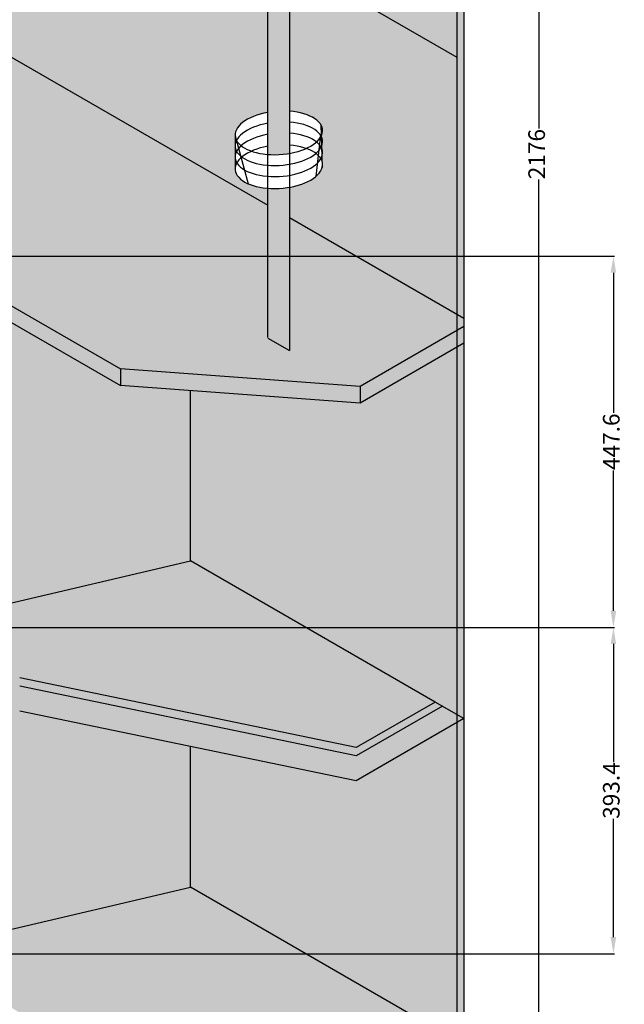
# Model space of a CAD drawing. Units: millimetres. Extents: x 78378 to 86415, y 148682 to 152721.
# Tile 11 of 18: x 81240 to 81968, y 149308 to 150495. Entities that reach past the tile are written whole.
import ezdxf

# ---------------------------------------------------------------- set-up
doc = ezdxf.new("R2010")
doc.units = ezdxf.units.MM
for name, color, linetype, lineweight in [('A-ANNO-DIMS', 2, 'Continuous', 18), ('A-FURN', 4, 'Continuous', 25), ('A-FURN-PATT', 32, 'Continuous', 13)]:
    doc.layers.add(name, color=color, linetype=linetype, lineweight=lineweight)
doc.styles.get("Standard").update_dxf_attribs({"font": 'arial.ttf'})
doc.dimstyles.new('ISO-25', dxfattribs={"dimtxt": 20, "dimasz": 20, "dimexe": 1.25, "dimexo": 0.625, "dimtad": 0, "dimdec": 1, "dimtxsty": 'Standard', "dimcen": 2.5, "dimadec": 0, "dimazin": 0, "dimtfac": 1, "dimtdec": 1, "dimtmove": 0, "dimatfit": 3, "dimfxl": 1, "dimarcsym": 0})

# ---------------------------------------------------------------- blocks, each defined once
blk = doc.blocks.new('*D1')
at = {"layer": 'A-ANNO-DIMS', "color": 0, "lineweight": -2, "transparency": 16777216}
for p, q in [((81775.8, 151435), (81866.6, 151435)), ((81865.3, 151415), (81865.3, 150363.7)), ((81865.3, 149279), (81865.3, 150302.4)), ((81775.8, 149259), (81866.6, 149259))]:
    blk.add_line(p, q, dxfattribs=at)
at = {"layer": 'A-ANNO-DIMS', "color": 0, "transparency": 16777216}
for points in [[(81862, 151415), (81868.6, 151415), (81865.3, 151435)], [(81862, 149279), (81868.6, 149279), (81865.3, 149259)]]:
    blk.add_solid(points, dxfattribs=at)
at = {"layer": 'Defpoints', "color": 0, "transparency": 16777216}
for p in [(81775.2, 151435), (81775.2, 149259), (81865.3, 149259)]:
    blk.add_point(p, dxfattribs=at)
at = {"layer": 'A-ANNO-DIMS', "color": 0, "transparency": 16777216, "insert": (81865.3, 150333), "char_height": 20, "attachment_point": 5, "rotation": 90}
blk.add_mtext('2176', dxfattribs=at)
blk = doc.blocks.new('*D28')
at = {"layer": 'A-ANNO-DIMS', "color": 0, "lineweight": -2, "transparency": 16777216}
for p, q in [((81117.6, 149762.4), (81956.4, 149762.4)), ((81955.2, 149742.4), (81955.2, 149600)), ((81955.2, 149389), (81955.2, 149531.4)), ((81117.6, 149369), (81956.4, 149369))]:
    blk.add_line(p, q, dxfattribs=at)
at = {"layer": 'A-ANNO-DIMS', "color": 0, "transparency": 16777216}
for points in [[(81951.8, 149742.4), (81958.5, 149742.4), (81955.2, 149762.4)], [(81951.8, 149389), (81958.5, 149389), (81955.2, 149369)]]:
    blk.add_solid(points, dxfattribs=at)
at = {"layer": 'Defpoints', "color": 0, "transparency": 16777216}
for p in [(81117, 149762.4), (81955.2, 149762.4), (81117, 149369)]:
    blk.add_point(p, dxfattribs=at)
at = {"layer": 'A-ANNO-DIMS', "color": 0, "transparency": 16777216, "insert": (81955.2, 149565.7), "char_height": 20, "attachment_point": 5, "rotation": 90}
blk.add_mtext('393.4', dxfattribs=at)
blk = doc.blocks.new('*D29')
at = {"layer": 'A-ANNO-DIMS', "color": 0, "lineweight": -2, "transparency": 16777216}
for p, q in [((81126.3, 150210), (81956.4, 150210)), ((81955.2, 150190), (81955.2, 150021)), ((81955.2, 149782.4), (81955.2, 149951.4)), ((81117.6, 149762.4), (81956.4, 149762.4))]:
    blk.add_line(p, q, dxfattribs=at)
at = {"layer": 'A-ANNO-DIMS', "color": 0, "transparency": 16777216}
for points in [[(81951.8, 150190), (81958.5, 150190), (81955.2, 150210)], [(81951.8, 149782.4), (81958.5, 149782.4), (81955.2, 149762.4)]]:
    blk.add_solid(points, dxfattribs=at)
at = {"layer": 'Defpoints', "color": 0, "transparency": 16777216}
for p in [(81125.6, 150210), (81955.2, 150210), (81117, 149762.4)]:
    blk.add_point(p, dxfattribs=at)
at = {"layer": 'A-ANNO-DIMS', "color": 0, "transparency": 16777216, "insert": (81955.2, 149986.2), "char_height": 20, "attachment_point": 5, "rotation": 90}
blk.add_mtext('447.6', dxfattribs=at)

msp = doc.modelspace()

# ---------------------------------------------------------------- hatches: boundary and pattern name
at = {"layer": 'A-FURN-PATT'}
h = msp.add_hatch(color=256, dxfattribs=at)
h.dxf.hatch_style = 1
h.paths.add_polyline_path([(78839.3276, 151040.0076), (78579.52, 151190.0076), (78579.52, 150470.0076), (78839.3276, 150320.0076)])
h.paths.add_polyline_path([(79073.1545, 150899.6469, 0.277779695), (79002.2645, 150996.3205, 0.791083931), (78917.9567, 150978.8719, 0.180448316), (78856.6481, 150853.0138), (78856.6481, 150350.6973), (79073.1545, 150484.318)])
h.paths.add_polyline_path([(79073.1545, 151175.0076), (78856.6481, 151050.0076), (78856.6481, 150853.0138, -0.180448316), (78917.9567, 150978.8719, -0.791083931), (79002.2645, 150996.3205, -0.277779695), (79073.1545, 150899.6469)])
h.paths.add_polyline_path([(79341.6224, 151350.0076), (79099.1352, 151490.0076), (78596.8405, 151200.0076), (78839.3276, 151060.0076)])
h.paths.add_polyline_path([(79904.5389, 151675.0076), (79662.0518, 151815.0076), (79099.1352, 151490.0076), (79341.6224, 151350.0076)])
h.paths.add_polyline_path([(80389.5131, 151955.0076), (80389.5131, 152235.0076), (79662.0518, 151815.0076), (79904.5389, 151675.0076)])
h.paths.add_polyline_path([(80389.5131, 151955.0076), (80164.3465, 151825.0076), (80164.3465, 151105.0076), (80614.6797, 151105.0076), (80614.6797, 151825.0076)])
edge = h.paths.add_edge_path(flags=16)
edge.add_spline(control_points=[(80216.308, 151728.251), (80227.1854, 151732.981), (80256.3301, 151745.6544), (80298.41, 151761.9595), (80340.2597, 151805.855), (80391.0771, 151782.0404), (80454.0396, 151805.7581), (80496.5007, 151742.4095), (80543.8218, 151733.4043), (80562.7182, 151729.8083)], knot_values=[0, 0, 0, 0, 35.543746761, 95.235753469, 136.367675126, 200.932981967, 236.726410811, 322.889934976, 380.170273667, 380.170273667, 380.170273667, 380.170273667], degree=3, periodic=0)
edge.add_line((80562.7182, 151729.8083), (80562.7182, 151165.0076))
edge.add_line((80562.7182, 151165.0076), (80216.308, 151165.0076))
edge.add_line((80216.308, 151165.0076), (80216.308, 151728.251))
h.paths.add_polyline_path([(80632.0002, 152095.0076), (80389.5131, 152235.0076), (80389.5131, 151955.0076), (80614.6797, 151825.0076), (80632.0002, 151815.0076)])
h.paths.add_polyline_path([(80867.7794, 151958.8805), (80632.0002, 152095.0076), (80632.0002, 151815.0076), (80632.0002, 151510.0076), (80867.7794, 151373.8805)])
h.paths.add_polyline_path([(80147.026, 151495.8203, 0.18918979), (80063.5671, 151597.7244, 0.788261355), (79979.2691, 151580.5832, 0.160726132), (79904.5389, 151413.5769), (79904.5389, 150955.0076), (80147.026, 151095.0076)])
h.paths.add_polyline_path([(80147.026, 151815.0076), (79904.5389, 151675.0076), (79904.5389, 151413.5769, -0.160726132), (79979.2691, 151580.5832, -0.788261355), (80063.5671, 151597.7244, -0.18918979), (80147.026, 151495.8203)])
h.paths.add_polyline_path([(79887.2184, 151645.0076), (79640.4011, 151502.5076), (79640.4011, 151262.3325, -0.160726132), (79715.1313, 151429.3387, -0.788261355), (79799.4294, 151446.48, -0.21290578), (79887.2184, 151328.7247)])
h.paths.add_polyline_path([(79799.4294, 151446.48, 0.788261355), (79715.1313, 151429.3387, 0.160726132), (79640.4011, 151262.3325), (79640.4011, 150822.5076), (79887.2184, 150965.0076), (79887.2184, 151328.7247, 0.21290578)])
h.paths.add_polyline_path([(79605.7601, 151482.5076), (79358.9429, 151340.0076), (79358.9429, 151100.0701, -0.160726132), (79433.6731, 151267.0764, -0.788261355), (79517.9711, 151284.2176, -0.21290578), (79605.7601, 151166.4623)])
h.paths.add_polyline_path([(79605.7601, 151166.4623, 0.21290578), (79517.9711, 151284.2176, 0.788261355), (79433.6731, 151267.0764, 0.160726132), (79358.9429, 151100.0701), (79358.9429, 150742.9831), (79419.0877, 150694.7323), (79605.7601, 150802.5076)])
edge = h.paths.add_edge_path(flags=0)
edge.add_spline(control_points=[(81152.4356, 151098.7676), (81105.7208, 151145.9466), (81038.6136, 151213.7208), (80882.3866, 151214.1938), (80797.4434, 151311.2997), (80711.8686, 151340.3754), (80681.7691, 151350.6023)], knot_values=[0, 0, 0, 0, 188.233441, 270.4032752, 445.451792012, 540.428588287, 540.428588287, 540.428588287, 540.428588287], degree=3, periodic=0)
edge.add_line((80683.4538, 151350.0269), (80683.4538, 151104.8792))
edge.add_line((80683.4538, 151104.8792), (81152.4356, 150851.399))
edge.add_line((81152.4356, 150851.399), (81152.4356, 151098.7676))
edge = h.paths.add_edge_path(flags=0)
edge.add_spline(control_points=[(80912.9018, 151027.1103), (80892.3742, 151034.1027), (80860.1663, 151045.0739), (80835.5097, 151068.1214), (80826.5679, 151076.4797)], knot_values=[0, 0, 0, 0, 63.98405104, 100.391424282, 100.391424282, 100.391424282, 100.391424282], degree=3, periodic=0)
edge.add_arc((80830.0414, 151081.2992), 5.9407, 100.9277276, 234.2187381, ccw=False)
edge.add_spline(control_points=[(80828.9152, 151087.1322), (80837.857, 151078.7739), (80862.5136, 151055.7263), (80894.7215, 151044.7552), (80915.2491, 151037.7628)], knot_values=[0, 0, 0, 0, 36.407373242, 100.391424282, 100.391424282, 100.391424282, 100.391424282], degree=3, periodic=0)
edge.add_arc((80914.7882, 151032.2795), 5.5026, -107.9540399, 85.195579, ccw=False)
h.paths.add_polyline_path([(81238.218, 151110.0076), (80632.0002, 151460.0076), (80632.0002, 151105.0076), (81238.218, 150755.0076)])
edge = h.paths.add_edge_path(flags=16)
edge.add_line((81152.4356, 150851.399), (80683.4538, 151104.8792))
edge.add_line((80683.4538, 151104.8792), (80683.4538, 151350.0279))
edge.add_spline(control_points=[(80681.7691, 151350.6023), (80711.8686, 151340.3754), (80797.4434, 151311.2997), (80882.3866, 151214.1938), (81038.6136, 151213.7208), (81105.7208, 151145.9466), (81152.4356, 151098.7676)], knot_values=[0, 0, 0, 0, 94.976796275, 270.025313088, 352.195147288, 540.428588287, 540.428588287, 540.428588287, 540.428588287], degree=3, periodic=0)
edge.add_line((81152.4356, 151098.7676), (81152.4356, 150851.399))
edge = h.paths.add_edge_path(flags=0)
edge.add_spline(control_points=[(80912.9018, 151027.1103), (80892.3742, 151034.1027), (80860.1663, 151045.0739), (80835.5097, 151068.1214), (80826.5679, 151076.4797)], knot_values=[0, 0, 0, 0, 63.98405104, 100.391424282, 100.391424282, 100.391424282, 100.391424282], degree=3, periodic=0)
edge.add_arc((80830.0414, 151081.2992), 5.9407, 100.9277276, 234.2187381, ccw=False)
edge.add_spline(control_points=[(80828.9152, 151087.1322), (80837.857, 151078.7739), (80862.5136, 151055.7263), (80894.7215, 151044.7552), (80915.2491, 151037.7628)], knot_values=[0, 0, 0, 0, 36.407373242, 100.391424282, 100.391424282, 100.391424282, 100.391424282], degree=3, periodic=0)
edge.add_arc((80914.7882, 151032.2795), 5.5026, -107.7417882, 85.195579, ccw=False)
h.paths.add_polyline_path([(81498.0256, 151255.0076), (81238.218, 151110.0076), (81238.218, 150755.0076), (81498.0256, 150905.0076)])
edge = h.paths.add_edge_path(flags=16)
edge.add_spline(control_points=[(81152.4356, 151098.7676), (81105.7208, 151145.9466), (81038.6136, 151213.7208), (80882.3866, 151214.1938), (80797.4434, 151311.2997), (80711.8686, 151340.3754), (80681.7691, 151350.6023)], knot_values=[0, 0, 0, 0, 188.233441, 270.4032752, 445.451792012, 540.428588287, 540.428588287, 540.428588287, 540.428588287], degree=3, periodic=0)
edge.add_line((80683.4538, 151350.0279), (80683.4538, 151104.8792))
edge.add_line((80683.4538, 151104.8792), (81152.4356, 150851.399))
edge.add_line((81152.4356, 150851.399), (81152.4356, 151098.7676))
h.paths.add_polyline_path([(81453.9904, 151280.4314), (80867.7794, 151618.8805), (80867.7794, 151373.8805), (81238.218, 151160.0076)])
edge = h.paths.add_edge_path(flags=16)
edge.add_line((81189.2304, 151297.6373), (81114.4166, 151300.2154))
edge.add_arc((81412.0967, 151394.0167), 312.1092, 179.7569303, 197.4900342, ccw=False)
edge.add_ellipse((81154.0183, 151392.0436), major_axis=(-54.0264, 3.6301), ratio=0.221796934, start_angle=0, end_angle=0.3517985, ccw=False)
edge.add_ellipse((81154.0183, 151392.0436), major_axis=(-54.0264, 3.6301), ratio=0.221796934, start_angle=180, end_angle=360, ccw=False)
edge.add_spline(control_points=[(81196.1844, 151321.9476), (81224.9802, 151347.1455), (81266.8846, 151383.8144), (81222.0354, 151387.0304), (81208.0056, 151388.0364)], knot_values=[0, 0, 0, 0, 75.091751734, 109.275804387, 109.275804387, 109.275804387, 109.275804387], degree=3, periodic=0)
edge.add_arc((80751.9112, 151435.6145), 458.5693, 342.4891602, 345.646172, ccw=False)
edge = h.paths.add_edge_path(flags=0)
edge.add_spline(control_points=[(81196.6193, 151323.657), (81197.893, 151324.7717), (81199.1654, 151325.8858), (81209.0233, 151334.5343), (81217.3959, 151341.9835), (81228.0928, 151352.5012), (81231.3883, 151355.9524), (81236.9493, 151362.4395), (81239.214, 151365.4773), (81241.4987, 151369.416), (81242.064, 151370.5542), (81242.9187, 151372.6971), (81243.2076, 151373.7015), (81243.5012, 151375.5539), (81243.5065, 151376.4), (81243.2432, 151377.9407), (81242.9775, 151378.6373), (81242.1402, 151379.937), (81241.5659, 151380.5416), (81240.2039, 151381.533), (81239.4963, 151381.9384), (81237.0619, 151383.0663), (81235.0242, 151383.6999), (81230.352, 151384.7569), (81227.7173, 151385.1826), (81221.9118, 151385.9145), (81218.7193, 151386.2133), (81213.7912, 151386.6115), (81212.1252, 151386.7359), (81209.6196, 151386.9181), (81208.7865, 151386.9779), (81207.9009, 151387.0432)], knot_values=[0.015487437, 0.015487437, 0.015487437, 0.015487437, 3.337879569, 3.337879569, 25.851306242, 25.851306242, 37.52811308, 37.52811308, 49.204919918, 49.204919918, 54.285093801, 54.285093801, 59.365267683, 59.365267683, 64.445441566, 64.445441566, 69.525615449, 69.525615449, 74.605789331, 74.605789331, 78.493667847, 78.493667847, 86.255670953, 86.255670953, 94.017674059, 94.017674059, 102.202265559, 102.202265559, 106.294561309, 106.294561309, 108.325221747, 108.325221747, 108.325221747, 108.325221747], degree=3, periodic=0)
edge = h.paths.add_edge_path(flags=16)
edge.add_arc((81034.1732, 151350.4693), 42.5822, 231.2679035, 306.151846, ccw=False)
edge.add_line((81007.5303, 151317.2517), (81007.5303, 151395.181))
edge.add_ellipse((81033.412, 151394.7791), major_axis=(-25.8816, 0.4538), ratio=0.23894509, start_angle=0, end_angle=0.1147075, ccw=False)
edge.add_ellipse((81033.412, 151394.7791), major_axis=(-25.8816, 0.4538), ratio=0.23894509, start_angle=181.1677709, end_angle=358.9476457, ccw=False)
edge.add_ellipse((81033.412, 151395.7791), major_axis=(-25.8816, 0.4538), ratio=0.23894509, start_angle=180, end_angle=360.1147075, ccw=False)
edge.add_ellipse((81033.412, 151395.7791), major_axis=(-25.8816, 0.4538), ratio=0.23894509, start_angle=178.9476457, end_angle=180, ccw=False)
edge.add_line((81059.2936, 151395.1778), (81059.2936, 151394.3772))
edge.add_ellipse((81033.412, 151394.7791), major_axis=(-25.8816, 0.4538), ratio=0.23894509, start_angle=180, end_angle=180.1147075, ccw=False)
edge.add_ellipse((81033.412, 151394.7791), major_axis=(-25.8816, 0.4538), ratio=0.23894509, start_angle=3.6903098, end_angle=176.4406503, ccw=False)
edge.add_line((81059.2936, 151393.3388), (81059.2936, 151316.086))
h.paths.add_polyline_path([(80951.9355, 151343.9568), (80909.6838, 151362.4635), (80904.0219, 151443.9615, -0.381333076), (80987.2169, 151411.3717)], flags=16)
h = msp.add_hatch(color=256, dxfattribs=at)
h.dxf.hatch_style = 1
h.paths.add_polyline_path([(80867.7794, 151978.8805), (80867.7794, 151958.8805), (81766.4935, 151440.0076), (81766.4935, 150140.0076), (81775.1537, 150135.0076), (81775.1537, 151455.0076)])
h = msp.add_hatch(color=256, dxfattribs=at)
h.dxf.hatch_style = 1
h.paths.add_polyline_path([(80389.8136, 150935.1811), (80389.5131, 151105.0076), (80164.3465, 151105.0076), (79904.5389, 150955.0076), (79433.5848, 150683.1022), (79459.4128, 150662.3818), (79243.9048, 150537.9582), (79160.4069, 150518.1674), (78839.3276, 150320.0076), (78579.52, 150470.0076), (78570.8597, 150475.0076), (78570.8597, 150465.0076), (78570.8597, 149885.0076)])
h.paths.add_polyline_path([(80086.4042, 150460.0076), (79826.5966, 150610.0076), (78570.8597, 149885.0076), (78830.6674, 149735.0076)])
h.paths.add_polyline_path([(79540.8001, 150161.0557), (79217.3967, 149974.3386), (78980.9166, 150110.8705), (79304.32, 150297.5875)], flags=16)
h.paths.add_polyline_path([(79506.159, 150161.0557), (79217.3967, 149994.3386), (79015.5576, 150110.8705), (79304.32, 150277.5875)], flags=0)
edge = h.paths.add_edge_path(flags=0)
edge.add_arc((79247.8636, 150177.1541), 137.9799, 256.0025928, 293.5594109)
edge.add_arc((79240.7671, 150078.2605), 68.0855, 336.099104, 387.3696877)
edge.add_ellipse((79258.3074, 150109.4852), major_axis=(-42.6234, -1.6591), ratio=0.160428429, start_angle=0, end_angle=179.0977279, ccw=False)
edge.add_arc((79285.2112, 150074.2509), 77.2096, 155.1233104, 203.6557939)
edge = h.paths.add_edge_path(flags=0)
edge.add_ellipse((79258.6958, 150110.8297), major_axis=(-42.6234, -1.6591), ratio=0.160428429, start_angle=350.6039412, end_angle=356.2289762)
edge.add_line((79219.169, 150111.8937), (79218.3268, 150109.4141))
edge.add_arc((79262.4675, 150032.9602), 88.2813, 112.3931229, 120, ccw=False)
h.paths.add_polyline_path([(79287.0625, 150086.9703, -0.247702064), (79288.1967, 150077.2955, -0.390476513), (79265.4731, 150072.5438, -0.487261526), (79264.079, 150082.3769, 0.395604326)], flags=0)
h.paths.add_polyline_path([(80389.5131, 150935.0076), (79826.5966, 150610.0076), (80086.4042, 150460.0076), (80692.622, 150460.0076), (80952.4296, 150610.0076)])
edge = h.paths.add_edge_path(flags=16)
edge.add_ellipse((80392.4466, 150825.601), major_axis=(-133.0757, 7.722), ratio=0.42449957, start_angle=0, end_angle=360)
edge = h.paths.add_edge_path(flags=0)
edge.add_spline(control_points=[(80269.3541, 150832.7436), (80269.2919, 150831.672), (80269.3503, 150830.5922), (80269.7341, 150828.3361), (80270.0612, 150827.1587), (80271.0461, 150824.6748), (80271.7052, 150823.3692), (80273.4061, 150820.6503), (80274.4481, 150819.2381), (80276.9366, 150816.3509), (80278.3828, 150814.8762), (80282.5858, 150811.0913), (80285.6261, 150808.7701), (80292.6031, 150804.2267), (80296.5388, 150802.0041), (80305.195, 150797.7581), (80309.9151, 150795.7344), (80320.0112, 150791.96), (80325.387, 150790.2092), (80339.2162, 150786.315), (80347.9578, 150784.3563), (80366.0679, 150781.2568), (80375.4359, 150780.1158), (80394.3093, 150778.7158), (80403.8142, 150778.4568), (80422.4656, 150778.8319), (80431.6115, 150779.4662), (80449.0608, 150781.5838), (80457.3636, 150783.0675), (80472.6699, 150786.7766), (80479.6726, 150789.0033), (80490.1894, 150793.2813), (80494.1268, 150795.1967), (80501.0146, 150799.1885), (80503.9632, 150801.2651), (80508.2066, 150804.9015), (80509.73, 150806.4609), (80512.1996, 150809.4942), (80513.1456, 150810.9657), (80514.4291, 150813.5431), (80514.8436, 150814.6688), (80515.3984, 150816.8625), (80515.5405, 150817.9315), (80515.5801, 150820.098), (80515.4773, 150821.1978), (80514.9905, 150823.5062), (80514.6047, 150824.7154), (80513.4854, 150827.2641), (80512.7511, 150828.6027), (80510.8872, 150831.3809), (80509.7578, 150832.8196), (80507.0873, 150835.7513), (80505.5466, 150837.2439), (80501.0624, 150841.0944), (80497.8199, 150843.4576), (80490.4174, 150848.062), (80486.2582, 150850.3037), (80477.1448, 150854.5643), (80472.1909, 150856.5835), (80461.6275, 150860.3245), (80456.0182, 150862.0465), (80441.7332, 150865.8127), (80432.7885, 150867.6675), (80414.3391, 150870.5317), (80404.8349, 150871.5411), (80385.7707, 150872.6572), (80376.2113, 150872.764), (80357.5444, 150872.0728), (80348.4375, 150871.2748), (80331.1682, 150868.83), (80323.0064, 150867.1827), (80309.472, 150863.5363), (80303.8628, 150861.6593), (80293.8018, 150857.5401), (80289.3512, 150855.2969), (80282.7757, 150851.2345), (80280.3473, 150849.4579), (80276.2606, 150845.9127), (80274.604, 150844.1458), (80272.3157, 150841.1243), (80271.5358, 150839.8454), (80270.3496, 150837.3879), (80269.9417, 150836.2101), (80269.5065, 150834.2815), (80269.3988, 150833.5143), (80269.3541, 150832.7436)], knot_values=[0, 0, 0, 0, 0.09750046, 0.09750046, 0.19500092, 0.19500092, 0.292501379, 0.292501379, 0.390001839, 0.390001839, 0.487502299, 0.487502299, 0.638803224, 0.638803224, 0.790104149, 0.790104149, 0.941405074, 0.941405074, 1.092705999, 1.092705999, 1.312817101, 1.312817101, 1.532928203, 1.532928203, 1.753039304, 1.753039304, 1.973150406, 1.973150406, 2.193261508, 2.193261508, 2.413372609, 2.413372609, 2.569860633, 2.569860633, 2.726348657, 2.726348657, 2.844186582, 2.844186582, 2.962024507, 2.962024507, 3.060233876, 3.060233876, 3.158443245, 3.158443245, 3.256652615, 3.256652615, 3.354861984, 3.354861984, 3.453071354, 3.453071354, 3.551280723, 3.551280723, 3.649490093, 3.649490093, 3.80392773, 3.80392773, 3.958365368, 3.958365368, 4.112803006, 4.112803006, 4.267240644, 4.267240644, 4.489203495, 4.489203495, 4.711166346, 4.711166346, 4.933129197, 4.933129197, 5.155092048, 5.155092048, 5.3770549, 5.3770549, 5.557853609, 5.557853609, 5.738652318, 5.738652318, 5.872395556, 5.872395556, 6.006138794, 6.006138794, 6.109604996, 6.109604996, 6.213071198, 6.213071198, 6.283185307, 6.283185307, 6.283185307, 6.283185307], degree=3, periodic=0)
edge = h.paths.add_edge_path(flags=0)
edge.add_ellipse((80392.4466, 150825.601), major_axis=(-101.8398, 3.3923), ratio=0.403492477, start_angle=0, end_angle=360)
edge = h.paths.add_edge_path(flags=0)
edge.add_ellipse((80391.1657, 150858.3746), major_axis=(9.0882, -0.6733), ratio=0.351354129, start_angle=0, end_angle=360)
h.paths.add_polyline_path([(80952.4296, 150610.0076), (80692.622, 150460.0076), (81361.2342, 150073.9842), (81649.9628, 150052.7286), (81766.4935, 150120.0076), (81766.4935, 150140.0076), (81564.9025, 150256.3963), (81564.8884, 150096.1963), (81538.9076, 150111.1963), (81538.9217, 150271.3963)])
h.paths.add_polyline_path([(81539.0357, 151571.3305), (80867.7794, 151958.8805), (80867.7794, 151618.8805), (81498.0256, 151255.0076), (81498.0256, 150905.0076), (81238.218, 150755.0076), (81538.9488, 150581.3806)])
h.paths.add_polyline_path([(81766.4935, 151440.0076), (81565.0164, 151556.3305), (81564.9296, 150566.3806), (81766.4935, 150450.0076)])
edge = h.paths.add_edge_path()
edge.add_line((81564.9296, 150566.3806), (81564.9137, 150384.6289))
edge.add_ellipse((81552.1304, 150358.5718), major_axis=(52.6272, 3.506), ratio=0.495899055, start_angle=367.5169757, end_angle=420.0564686, ccw=False)
edge.add_ellipse((81552.1304, 150358.5718), major_axis=(52.6272, 3.506), ratio=0.495899055, start_angle=351.729742, end_angle=367.5169757, ccw=False)
edge.add_ellipse((81552.1304, 150345.5016), major_axis=(52.6272, 3.506), ratio=0.495899055, start_angle=352.5116949, end_angle=366.3006092, ccw=False)
edge.add_line((81603.4463, 150342.2039), (81603.5064, 150340.4475))
edge.add_ellipse((81552.1304, 150332.128), major_axis=(52.6272, 3.506), ratio=0.495899055, start_angle=353.6729654, end_angle=365.3867997, ccw=False)
edge.add_ellipse((81552.1304, 150332.128), major_axis=(52.6272, 3.506), ratio=0.495899055, start_angle=350.9388331, end_angle=353.6729654)
edge.add_line((81603.8688, 150329.855), (81604.0442, 150324.7302))
edge.add_ellipse((81552.1304, 150317.7418), major_axis=(52.6272, 3.506), ratio=0.495899055, start_angle=355.2176746, end_angle=363.8553364, ccw=False)
edge.add_ellipse((81552.1304, 150317.7418), major_axis=(52.6272, 3.506), ratio=0.495899055, start_angle=341.3250873, end_angle=355.2176746, ccw=False)
edge.add_ellipse((81552.1304, 150317.7418), major_axis=(52.6272, 3.506), ratio=0.495899055, start_angle=293.4661701, end_angle=341.3250873, ccw=False)
edge.add_line((81564.9057, 150292.9664), (81564.9025, 150256.3963))
edge.add_line((81564.9025, 150256.3963), (81766.4935, 150140.0076))
edge.add_line((81766.4935, 150140.0076), (81766.4935, 150450.0076))
edge.add_line((81766.4935, 150450.0076), (81564.9296, 150566.3806))
h.paths.add_polyline_path([(81525.5713, 150321.598), (81526.5985, 150321.3069), (81528.6771, 150320.947)])
h.paths.add_polyline_path([(81512.7903, 150326.1129), (81514.5058, 150325.3887), (81512.538, 150326.2678)])
h.paths.add_polyline_path([(81533.2148, 150320.1615), (81534.6952, 150319.9052), (81536.5995, 150319.7557)])
h.paths.add_polyline_path([(81518.622, 150323.6513), (81519.227, 150323.3959), (81521.289, 150322.8116)])
h.paths.add_polyline_path([(81501.2183, 150336.2599), (81500.3543, 150338.1339), (81499.7815, 150340.0494), (81499.5032, 150341.9955), (81499.5032, 150343.7257), (81499.7584, 150345.5905), (81500.2766, 150347.4549), (81501.0551, 150349.3095), (81501.0967, 150349.3937), (81501.1389, 150349.4778), (81500.9978, 150349.7496), (81500.8628, 150350.0225), (81499.5032, 150355.0658), (81499.9591, 150359.5002), (81501.8982, 150363.9083), (81505.2653, 150368.1646), (81509.9647, 150372.1482), (81515.8627, 150375.7459), (81522.7918, 150378.8553), (81530.555, 150381.3882), (81538.9315, 150383.2724), (81538.9488, 150581.3806), (80632.0002, 151105.0076), (80389.5131, 151105.0076), (80389.8142, 150934.8338), (80952.4296, 150610.0076), (81538.9217, 150271.3963), (81538.9234, 150291.7194), (81538.8752, 150291.721), (81530.1915, 150292.8239), (81522.1802, 150294.6904), (81515.0866, 150297.2633), (81509.8635, 150299.9959), (81505.6084, 150303.1351), (81502.419, 150306.6088), (81500.3683, 150310.3375), (81499.5032, 150314.2358), (81499.5032, 150315.9659), (81499.8206, 150318.1159), (81500.487, 150320.2634), (81501.4979, 150322.3941), (81500.487, 150324.4233), (81499.8206, 150326.5039), (81499.5032, 150328.622), (81499.5032, 150330.3521), (81499.7815, 150332.3262), (81500.3543, 150334.2992)])
h = msp.add_hatch(color=256, dxfattribs=at)
h.dxf.hatch_style = 1
h.paths.add_polyline_path([(79090.475, 151205.0076), (78839.3276, 151060.0076), (78839.3276, 150320.0076), (79090.475, 150475.0076)])
h.paths.add_polyline_path([(79073.1545, 151175.0076), (79073.1545, 150899.6469, -0.04544363), (79073.1545, 150878.5653), (79073.1545, 150484.318), (78856.6481, 150350.6973), (78856.6481, 150814.5249, -0.048157161), (78856.6481, 150853.0138), (78856.6481, 151050.0076)], flags=16)
h.paths.add_polyline_path([(79358.9429, 151340.0076), (79605.7601, 151482.5076), (79605.7601, 150802.5076), (79419.0877, 150694.7323), (79433.5848, 150683.1022), (79623.0806, 150792.5076), (79623.0806, 151512.5076), (79341.6224, 151350.0076), (79341.6224, 150756.8784), (79358.9429, 150742.9831)])
h.paths.add_polyline_path([(79341.6224, 151350.0076), (79090.475, 151205.0076), (79090.475, 150475.0076), (79160.4069, 150518.1674), (79107.7955, 150505.6973), (79107.7955, 151195.0076), (79109.5275, 151196.0076), (79324.3018, 151320.0076), (79324.3018, 150770.7736), (79341.6224, 150756.8784)])
h.paths.add_polyline_path([(79887.2184, 151645.0076), (79887.2184, 151665.0076), (79623.0806, 151512.5076), (79623.0806, 150792.5076), (79887.2184, 150945.0076), (79887.2184, 150965.0076), (79640.4011, 150822.5076), (79640.4011, 151502.5076)])
h.paths.add_polyline_path([(79904.5389, 151655.0076), (79887.2184, 151645.0076), (79887.2184, 150965.0076), (79904.5389, 150975.0076)])
h.paths.add_polyline_path([(80164.3465, 151825.0076), (80147.026, 151815.0076), (80147.026, 151095.0076), (80164.3465, 151105.0076)])
h.paths.add_polyline_path([(80632.0002, 151510.0076), (80632.0002, 151490.0076), (81238.218, 151140.0076), (81471.6045, 151270.2619), (81453.9904, 151280.4314), (81238.218, 151160.0076)])
h.paths.add_polyline_path([(80632.0002, 151490.0076), (80632.0002, 151470.0076), (81238.218, 151120.0076), (81489.2186, 151260.0924), (81471.6045, 151270.2619), (81238.218, 151140.0076)])
h.paths.add_polyline_path([(80632.0002, 151460.0076), (80632.0002, 151105.0076), (81238.218, 150755.0076), (81238.218, 151110.0076)])
edge = h.paths.add_edge_path(flags=16)
edge.add_spline(control_points=[(80681.7691, 151350.6023), (80711.8686, 151340.3754), (80797.4434, 151311.2997), (80882.3866, 151214.1938), (81038.6136, 151213.7208), (81105.7208, 151145.9466), (81152.4356, 151098.7676)], knot_values=[0, 0, 0, 0, 94.976796275, 270.025313088, 352.195147288, 540.428588287, 540.428588287, 540.428588287, 540.428588287], degree=3, periodic=0)
edge.add_line((81152.4356, 151098.7676), (81152.4356, 150851.399))
edge.add_line((81152.4356, 150851.399), (80683.4538, 151104.8792))
edge.add_line((80683.4538, 151104.8792), (80683.4538, 151350.027))
edge = h.paths.add_edge_path(flags=0)
edge.add_spline(control_points=[(80828.9152, 151087.1322), (80837.857, 151078.7739), (80862.5136, 151055.7263), (80894.7215, 151044.7552), (80915.2491, 151037.7628)], knot_values=[0, 0, 0, 0, 36.407373242, 100.391424282, 100.391424282, 100.391424282, 100.391424282], degree=3, periodic=0)
edge.add_arc((80914.7882, 151032.2795), 5.5026, -107.9540399, 85.195579, ccw=False)
edge.add_spline(control_points=[(80912.9018, 151027.1103), (80892.3742, 151034.1027), (80860.1663, 151045.0739), (80835.5097, 151068.1214), (80826.5679, 151076.4797)], knot_values=[0, 0, 0, 0, 63.98405104, 100.391424282, 100.391424282, 100.391424282, 100.391424282], degree=3, periodic=0)
edge.add_arc((80830.0414, 151081.2992), 5.9407, 100.9277276, 234.2187381, ccw=False)
h.paths.add_polyline_path([(80632.0002, 151815.0076), (80614.6797, 151825.0076), (80614.6797, 151105.0076), (80632.0002, 151105.0076)])
h.paths.add_polyline_path([(81498.0256, 151255.0076), (81489.2186, 151260.0924), (81238.218, 151120.0076), (80632.0002, 151470.0076), (80632.0002, 151460.0076), (81238.218, 151110.0076)])
h.paths.add_polyline_path([(78596.8405, 151200.0076), (78579.52, 151190.0076), (78839.3276, 151040.0076), (78839.3276, 151060.0076)])
h.paths.add_polyline_path([(78596.8405, 151200.0076), (78579.52, 151210.0076), (78579.52, 151190.0076)])
h.paths.add_polyline_path([(78579.52, 151210.0076), (78570.8597, 151205.0076), (78570.8597, 150475.0076), (78579.52, 150470.0076)])
h = msp.add_hatch(color=256, dxfattribs=at)
h.dxf.hatch_style = 1
edge = h.paths.add_edge_path()
edge.add_line((81565.0164, 151556.3305), (81539.0357, 151571.3305))
edge.add_line((81539.0357, 151571.3305), (81538.927, 150332.5469))
edge.add_ellipse((81552.1304, 150358.5718), major_axis=(52.6272, 3.506), ratio=0.495899055, start_angle=239.2882719, end_angle=293.4732997)
edge.add_line((81564.9092, 150333.797), (81565.0164, 151556.3305))
edge = h.paths.add_edge_path()
edge.add_ellipse((81552.1304, 150317.7418), major_axis=(52.6272, 3.506), ratio=0.495899055, start_angle=239.2817509, end_angle=293.4661701, ccw=False)
edge.add_line((81538.9234, 150291.7172), (81538.9076, 150111.1963))
edge.add_line((81538.9076, 150111.1963), (81564.8884, 150096.1963))
edge.add_line((81564.8884, 150096.1963), (81564.9057, 150292.9664))
h = msp.add_hatch(color=256, dxfattribs=at)
h.dxf.hatch_style = 1
h.paths.add_polyline_path([(81239.9694, 149691.4023), (81125.6347, 149757.4135), (81125.6347, 149727.4135), (81239.9694, 149661.4023), (81645.2499, 149577.4135), (81670.0493, 149591.7314), (81766.4935, 149647.4135), (81766.4935, 149657.4135), (81749.173, 149667.4135), (81645.2499, 149607.4135)])
h.paths.add_polyline_path([(81239.9694, 149701.4023), (81125.6347, 149767.4135), (81125.6347, 149757.4135), (81239.9694, 149691.4023), (81645.2499, 149607.4135), (81749.173, 149667.4135), (81740.5127, 149672.4135), (81645.2499, 149617.4135)])
h.paths.add_polyline_path([(81116.9744, 150195.0076), (80692.622, 150440.0076), (80692.622, 149614.0076), (81116.9744, 149369.0076)])
h.paths.add_polyline_path([(81073.6732, 149444.0076), (80735.9233, 149639.0076), (80735.9233, 150365.0076), (81073.6732, 150170.0076)], flags=16)
h.paths.add_polyline_path([(81125.6347, 149727.4135), (81116.9744, 149732.4135), (81116.9744, 149369.0076), (81239.9694, 149297.9965), (81239.9694, 149307.9965), (81125.6347, 149374.0076)])
h.paths.add_polyline_path([(81445.5517, 150047.7769), (81361.2342, 150053.9842), (81125.6347, 150190.0076), (81125.6347, 149767.4135), (81445.5517, 149842.7093)])
h.paths.add_polyline_path([(81239.9694, 149307.9965), (81239.9694, 149297.9965), (81645.2499, 149214.0076), (81645.2499, 149224.0076)])
h.paths.add_polyline_path([(81749.173, 149274.0076), (81740.5127, 149279.0076), (81645.2499, 149224.0076), (81645.2499, 149214.0076)])
h = msp.add_hatch(color=256, dxfattribs=at)
h.dxf.hatch_style = 1
h.paths.add_polyline_path([(81125.6347, 150210.0076), (81125.6347, 150190.0076), (81361.2342, 150053.9842), (81361.2342, 150073.9842)])
h.paths.add_polyline_path([(81361.2342, 150073.9842), (81361.2342, 150053.9842), (81649.9628, 150032.7286), (81649.9628, 150052.7286)])
h.paths.add_polyline_path([(81766.4935, 150100.0076), (81766.4935, 150120.0076), (81649.9628, 150052.7286), (81649.9628, 150032.7286)])
h.paths.add_polyline_path([(81775.1537, 150125.0076), (81766.4935, 150120.0076), (81766.4935, 150100.0076), (81775.1537, 150105.0076)])
h.paths.add_polyline_path([(81775.1537, 150135.0076), (81766.4935, 150140.0076), (81766.4935, 150120.0076), (81775.1537, 150125.0076)])
h = msp.add_hatch(color=256, dxfattribs=at)
h.dxf.hatch_style = 1
h.paths.add_polyline_path([(81445.5517, 150047.7769), (81361.2342, 150053.9842), (81125.6347, 150190.0076), (81125.6347, 149767.4135), (81445.5517, 149842.7093)])
h.paths.add_polyline_path([(81766.4935, 150100.0076), (81649.9628, 150032.7286), (81445.5517, 150047.7769), (81445.5517, 149842.7093), (81740.5127, 149672.4135), (81766.4935, 149657.4135)])
h.paths.add_polyline_path([(81445.5517, 149842.7093), (81125.6347, 149767.4135), (81239.9694, 149701.4023), (81645.2499, 149617.4135), (81740.5127, 149672.4135)])
h = msp.add_hatch(color=256, dxfattribs=at)
h.dxf.hatch_style = 1
h.paths.add_polyline_path([(81775.1537, 150105.0076), (81766.4935, 150100.0076), (81766.4935, 149657.4135), (81775.1537, 149652.4135)])
h.paths.add_polyline_path([(81775.1537, 149652.4135), (81766.4935, 149647.4135), (81766.4935, 149264.0076), (81775.1537, 149259.0076)])
h.paths.add_polyline_path([(81766.4935, 149657.4135), (81766.4935, 149647.4135), (81775.1537, 149652.4135)])
h = msp.add_hatch(color=256, dxfattribs=at)
h.dxf.hatch_style = 1
h.paths.add_polyline_path([(81445.5517, 149618.7982), (81239.9694, 149661.4023), (81125.6347, 149727.4135), (81125.6347, 149374.0076), (81445.5517, 149449.3035)])
h.paths.add_polyline_path([(81766.4935, 149647.4135), (81670.0493, 149591.7314), (81645.2499, 149577.4135), (81445.5517, 149618.7982), (81445.5517, 149449.3035), (81740.5127, 149279.0076), (81766.4935, 149264.0076)])
h.paths.add_polyline_path([(81445.5517, 149449.3035), (81125.6347, 149374.0076), (81239.9694, 149307.9965), (81645.2499, 149224.0076), (81740.5127, 149279.0076)])
h.paths.add_polyline_path([(81239.9694, 149297.9965), (81239.9694, 149267.9965), (81645.2499, 149184.0076), (81645.2499, 149214.0076)])

# ---------------------------------------------------------------- linework, layer by layer
at = {"layer": 'A-FURN'}
for p, q in [((81538.9076, 150111.7066), (81539.0357, 151571.3305)), ((81565.0164, 151556.3305), (81564.8884, 150096.1963)), ((81775.1537, 151455.0076), (81775.1537, 149259.0076)), ((81766.4935, 151440.0076), (81766.4935, 149264.0076)), ((80389.5131, 150935.0076), (81538.9076, 150271.4044)), ((81564.9296, 150566.3806), (81766.4935, 150450.0076)), ((80692.622, 150460.0076), (81361.2342, 150073.9842)), ((80692.622, 150440.0076), (81361.2342, 150053.9842)), ((81602.5408, 150368.6708), (81604.3135, 150316.8575)), ((81499.5032, 150355.0658), (81515.0866, 150297.2633)), ((81499.5032, 150355.0658), (81499.5032, 150314.2358)), ((81602.2067, 150356.1143), (81596.5965, 150305.9406)), ((81564.8884, 150256.4044), (81775.1537, 150135.0076)), ((81775.1537, 150125.0076), (81649.9628, 150052.7286)), ((81538.8812, 150111.2116), (81564.8884, 150096.1963)), ((81775.1537, 150105.0076), (81649.9628, 150032.7286)), ((81649.9628, 150052.7286), (81361.2342, 150073.9842)), ((81361.2342, 150073.9842), (81361.2342, 150053.9842)), ((81649.9628, 150032.7286), (81361.2342, 150053.9842)), ((81649.9628, 150052.7286), (81649.9628, 150032.7286)), ((81445.5517, 149842.7093), (81445.5517, 150047.7769)), ((81125.6347, 149767.4135), (81445.5517, 149842.7093)), ((81740.5127, 149672.4135), (81445.5517, 149842.7093)), ((81645.2499, 149617.4135), (81239.9694, 149701.4023)), ((81645.2499, 149607.4135), (81239.9694, 149691.4023)), ((81740.5127, 149672.4135), (81645.2499, 149617.4135)), ((81775.1537, 149652.4135), (81740.5127, 149672.4135)), ((81645.2499, 149577.4135), (81239.9694, 149661.4023)), ((81749.173, 149667.4135), (81645.2499, 149607.4135)), ((81749.173, 149667.4135), (81645.2499, 149607.4135)), ((81775.1537, 149652.4135), (81645.2499, 149577.4135)), ((81775.1537, 149652.4135), (81670.0493, 149591.7314)), ((81445.5517, 149449.3035), (81445.5517, 149618.7982)), ((81670.0493, 149591.7314), (81645.2499, 149577.4135)), ((81125.6347, 149374.0076), (81445.5517, 149449.3035)), ((81740.5127, 149279.0076), (81445.5517, 149449.3035))]:
    msp.add_line(p, q, dxfattribs=at)
for centre, start_param, end_param in [((81552.1304, 150358.5718), 1.791136933, 7.575735705), ((81552.1304, 150345.5016), 1.791159425, 7.575758142), ((81552.1304, 150332.128), 1.791182439, 7.575781099), ((81552.1304, 150317.7418), 1.791207196, 7.575805795)]:
    msp.add_ellipse(centre, major_axis=(52.6272, 3.506), ratio=0.495899055, start_param=start_param, end_param=end_param, dxfattribs=at)

# ---------------------------------------------------------------- dimensions: what is measured, and where the dimension line sits
at = {"layer": 'A-ANNO-DIMS'}
dim = msp.add_linear_dim(base=(81865.3079, 149259.0076), p1=(81775.1537, 151435.0076), p2=(81775.1537, 149259.0076), angle=270, dimstyle='ISO-25', override={"dimclrd": 0, "dimclre": 0, "dimclrt": 0}, dxfattribs=at)
dim.commit()
dim.dimension.update_dxf_attribs({"geometry": '*D1', "text_midpoint": (81865.3079, 150333.0085), "dimtype": 161})
for base, p1, p2, picture, middle in [((81955.1537, 150210.0076), (81116.9744, 149762.4135), (81125.6347, 150210.0076), '*D29', (81955.1537, 149986.2106)), ((81955.1537, 149762.4135), (81116.9744, 149369.0076), (81116.9744, 149762.4135), '*D28', (81955.1537, 149565.7106))]:
    dim = msp.add_linear_dim(base=base, p1=p1, p2=p2, angle=90, dimstyle='ISO-25', override={"dimdec": 1, "dimlfac": 1, "dimrnd": 0, "dimzin": 0, "dimdsep": 46, "dimlunit": 2}, dxfattribs=at)
    dim.commit()
    dim.dimension.update_dxf_attribs({"geometry": picture, "text_midpoint": middle})

doc.saveas('drawing.dxf')
